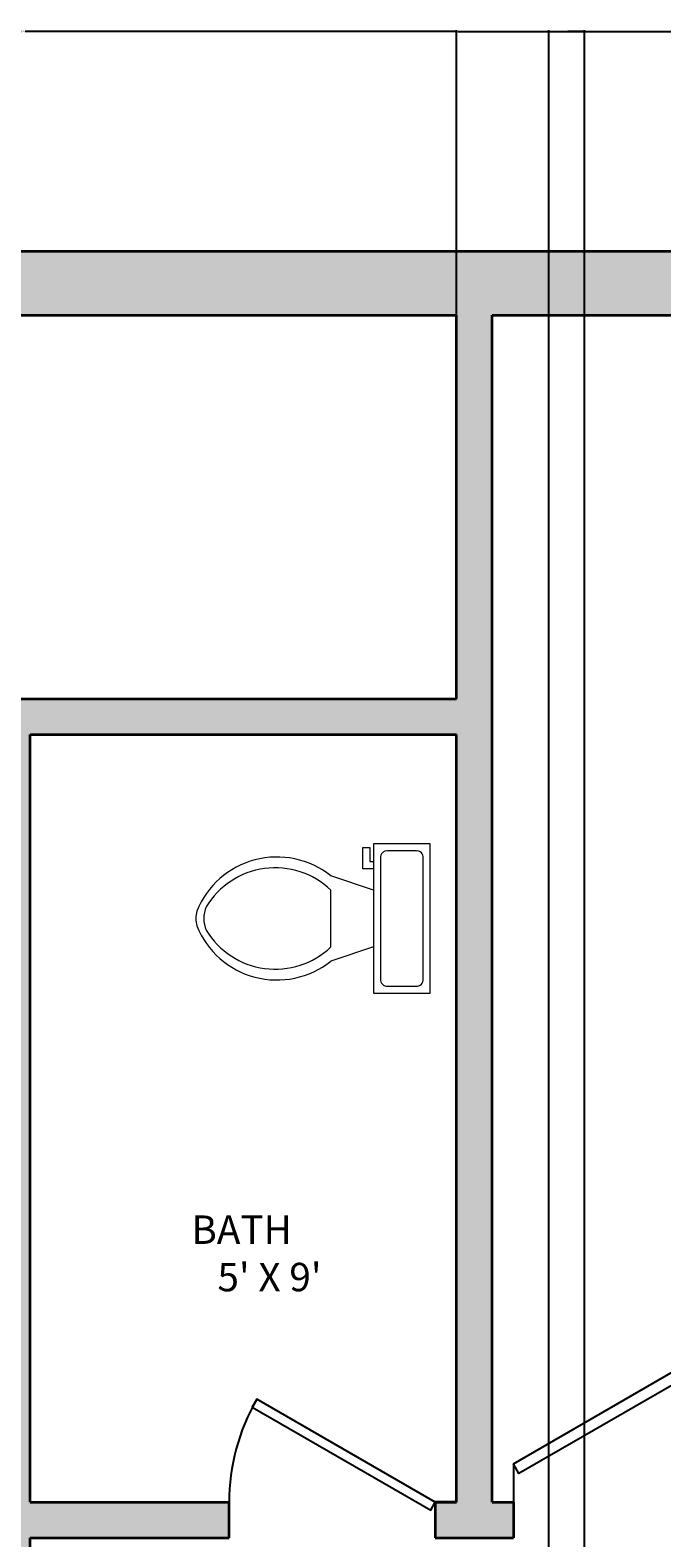
# Model space of a CAD drawing. Units: inches. Extents: x -30 to 437, y -29 to 647.
# Tile 14 of 15: x 187 to 276, y 435 to 647. Entities that reach past the tile are written whole.
import ezdxf

# ---------------------------------------------------------------- set-up
doc = ezdxf.new("R2010")
doc.units = ezdxf.units.IN
doc.header["$MEASUREMENT"] = 0
for name, color, linetype, lineweight in [('A-ANNO-DIMS', 2, 'Continuous', 18), ('A-AREA-IDEN', 7, 'Continuous', 18), ('A-WALL', 7, 'Continuous', 35), ('bathroom', 90, 'Continuous', 18), ('doors', 40, 'Continuous', 25)]:
    doc.layers.add(name, color=color, linetype=linetype, lineweight=lineweight)
doc.layers.add('A-WALL-PATT', color=251, linetype='Continuous', lineweight=13, true_color=0x636466)
doc.styles.get("Standard").update_dxf_attribs({"font": 'arial.ttf'})
doc.dimstyles.get("Standard").update_dxf_attribs({"dimtxt": 0.18, "dimasz": 0.18, "dimexe": 0.18, "dimexo": 0.0625, "dimgap": 0.09, "dimtad": 0, "dimtih": 1, "dimtoh": 1, "dimdec": 4, "dimzin": 0, "dimdsep": 46, "dimtxsty": 'Standard', "dimcen": 0.09, "dimadec": 0, "dimazin": 0, "dimtfac": 1, "dimtdec": 4, "dimtofl": 0, "dimtmove": 0, "dimatfit": 3, "dimfxl": 1, "dimtolj": 1, "dimtzin": 0, "dimarcsym": 0})

# ---------------------------------------------------------------- blocks, each defined once
blk = doc.blocks.new('Toilet - top')
for p, q in [((9.5, -6), (9.5, -2)), ((-8, -8.5), (-8, -8)), ((-7, -8), (-7, -9.5)), ((-4, -8), (-6, -14)), ((4, -8), (6, -14)), ((-10, -8.5), (-8, -8.5)), ((-10, -9.5), (-10, -8.5)), ((-7, -9.5), (-10, -9.5)), ((4, -14), (-4, -14))]:
    blk.add_line(p, q)
blk.add_lwpolyline([(10.5, -8), (10.5, 0), (-10.5, 0), (-10.5, -8)], close=True)
for points in [[(-9.5, -2), (-9.5, -6)], [(8.5, -1), (-8.5, -1)], [(-8.5, -7), (8.5, -7)]]:
    blk.add_lwpolyline(points)
for centre, radius, start, end in [((-8.62, -1.88), 0.884, 81.8699, 188.1301), ((8.62, -1.88), 0.884, 351.8699, 98.1301), ((-8.62, -6.12), 0.884, 171.8699, 278.1301), ((8.62, -6.12), 0.884, 261.8699, 8.1301), ((3.52, -21.58), 12.17, 141.4691, 247.9714), ((4.2, -21.82), 11.33, 136.3677, 238.9468), ((-3.52, -21.58), 12.17, 292.0284, 38.5307), ((-4.2, -21.82), 11.33, 301.053, 43.6321), ((0, -27.88), 4, 245.7318, 294.2682), ((0, -29), 4, 254.8605, 285.1395)]:
    blk.add_arc(centre, radius, start, end)
blk = doc.blocks.new('*U6')
for p, q in [((0, 0), (0, -6)), ((40, 0), (40, -6))]:
    blk.add_line(p, q)
blk.add_lwpolyline([(0, 0), (34.64, 20), (35.52, 18.48), (0.87, -1.52)], close=True)
blk.add_arc((0, 0), 40, 0, 30)
blk = doc.blocks.new('*U7')
for p, q in [((0, 0), (0, 6)), ((40, 0), (40, 6))]:
    blk.add_line(p, q)
blk.add_lwpolyline([(0, 0), (34.64, -20), (35.52, -18.48), (0.87, 1.52)], close=True)
blk.add_arc((0, 0), 40, 330, 0)
blk = doc.blocks.new('*D28')
at = {"layer": 'A-ANNO-DIMS', "color": 0, "lineweight": -2, "transparency": 16777216}
for p, q in [((124.67, 606.61), (124.67, 646.63)), ((124.85, 646.45), (185.39, 646.45)), ((246.49, 646.45), (185.95, 646.45)), ((246.67, 606.61), (246.67, 646.63))]:
    blk.add_line(p, q, dxfattribs=at)
at = {"layer": 'A-ANNO-DIMS', "color": 0, "transparency": 16777216}
for points in [[(124.85, 646.48), (124.85, 646.42), (124.67, 646.45)], [(246.49, 646.48), (246.49, 646.42), (246.67, 646.45)]]:
    blk.add_solid(points, dxfattribs=at)
at = {"layer": 'Defpoints', "color": 0, "transparency": 16777216}
for p in [(246.67, 646.45), (124.67, 606.55), (246.67, 606.55)]:
    blk.add_point(p, dxfattribs=at)
at = {"layer": 'A-ANNO-DIMS', "color": 0, "transparency": 16777216, "insert": (185.67, 646.45), "char_height": 0.18, "attachment_point": 5}
blk.add_mtext('\\A1;122', dxfattribs=at)
blk = doc.blocks.new('*D29')
at = {"layer": 'A-ANNO-DIMS', "color": 0, "lineweight": -2, "transparency": 16777216}
for p, q in [((246.67, 606.61), (246.67, 646.63)), ((246.85, 646.45), (325.89, 646.45)), ((405.49, 646.45), (326.45, 646.45)), ((405.67, 615.61), (405.67, 646.63))]:
    blk.add_line(p, q, dxfattribs=at)
at = {"layer": 'A-ANNO-DIMS', "color": 0, "transparency": 16777216}
for points in [[(246.85, 646.48), (246.85, 646.42), (246.67, 646.45)], [(405.49, 646.48), (405.49, 646.42), (405.67, 646.45)]]:
    blk.add_solid(points, dxfattribs=at)
at = {"layer": 'Defpoints', "color": 0, "transparency": 16777216}
for p in [(405.67, 646.45), (405.67, 615.55), (246.67, 606.55)]:
    blk.add_point(p, dxfattribs=at)
at = {"layer": 'A-ANNO-DIMS', "color": 0, "transparency": 16777216, "insert": (326.17, 646.45), "char_height": 0.18, "attachment_point": 5}
blk.add_mtext('\\A1;159', dxfattribs=at)
blk = doc.blocks.new('*D54')
at = {"layer": 'A-ANNO-DIMS', "color": 0, "lineweight": -2, "transparency": 16777216}
for p, q in [((259.67, 254.61), (259.67, 646.63)), ((259.85, 646.45), (262.02, 646.45)), ((264.49, 646.45), (262.32, 646.45)), ((264.67, 249.61), (264.67, 646.63))]:
    blk.add_line(p, q, dxfattribs=at)
at = {"layer": 'A-ANNO-DIMS', "color": 0, "transparency": 16777216}
for points in [[(259.85, 646.48), (259.85, 646.42), (259.67, 646.45)], [(264.49, 646.48), (264.49, 646.42), (264.67, 646.45)]]:
    blk.add_solid(points, dxfattribs=at)
at = {"layer": 'Defpoints', "color": 0, "transparency": 16777216}
for p in [(259.67, 646.45), (259.67, 254.55), (264.67, 249.55)]:
    blk.add_point(p, dxfattribs=at)
at = {"layer": 'A-ANNO-DIMS', "color": 0, "transparency": 16777216, "insert": (262.17, 646.45), "char_height": 0.18, "attachment_point": 5}
blk.add_mtext('\\A1;5', dxfattribs=at)

msp = doc.modelspace()

# ---------------------------------------------------------------- hatches: boundary and pattern name
at = {"layer": 'A-WALL-PATT'}
h = msp.add_hatch(color=256, dxfattribs=at)
h.dxf.hatch_style = 1
h.paths.add_polyline_path([(393.6054, 183.2352), (369.6054, 183.2352), (369.6054, 213.2352), (393.6054, 213.2352), (393.6054, 207.2352), (394.6054, 207.2352), (394.6054, 211.2352), (395.6054, 211.2352), (395.6054, 185.2352), (394.6054, 185.2352), (394.6054, 189.2352), (393.6054, 189.2352)], flags=0)
h.paths.add_polyline_path([(384.6054, 189.2352, -1), (390.6054, 189.2352, -1)], flags=0)
h.paths.add_polyline_path([(385.6054, 189.2352, -1), (389.6054, 189.2352, -1)], flags=0)
h.paths.add_polyline_path([(374.6054, 189.2352, -1), (382.6054, 189.2352, -1)], flags=0)
h.paths.add_polyline_path([(386.6054, 189.2352, -1), (388.6054, 189.2352, -1)], flags=0)
h.paths.add_polyline_path([(375.6054, 189.2352, -1), (381.6054, 189.2352, -1)], flags=0)
h.paths.add_polyline_path([(376.6054, 189.2352, -1), (380.6054, 189.2352, -1)], flags=0)
h.paths.add_polyline_path([(377.6054, 189.2352, -1), (379.6054, 189.2352, -1)], flags=0)
h.paths.add_polyline_path([(390.6054, 195.2352), (374.6054, 195.2352), (374.6054, 201.2352), (390.6054, 201.2352)], flags=0)
h.paths.add_polyline_path([(389.6054, 196.2352), (375.6054, 196.2352), (375.6054, 200.2352), (389.6054, 200.2352)], flags=0)
h.paths.add_polyline_path([(383.6054, 207.2352, -1), (391.6054, 207.2352, -1)], flags=0)
h.paths.add_polyline_path([(384.6054, 207.2352, -1), (390.6054, 207.2352, -1)], flags=0)
h.paths.add_polyline_path([(385.6054, 207.2352, -1), (389.6054, 207.2352, -1)], flags=0)
h.paths.add_polyline_path([(386.6054, 207.2352, -1), (388.6054, 207.2352, -1)], flags=0)
h.paths.add_polyline_path([(375.6054, 207.2352, -1), (381.6054, 207.2352, -1)], flags=0)
h.paths.add_polyline_path([(376.6054, 207.2352, -1), (380.6054, 207.2352, -1)], flags=0)
h.paths.add_polyline_path([(377.6054, 207.2352, -1), (379.6054, 207.2352, -1)], flags=0)
h.paths.add_polyline_path([(305.5437, 160.3663, -0.41421356), (304.0437, 158.8663), (271.0437, 158.8663, -0.41421356), (269.5437, 160.3663), (269.5437, 178.3663, -0.41421356), (271.0437, 179.8663), (304.0437, 179.8663, -0.41421356), (305.5437, 178.3663)], flags=0)
h.paths.add_polyline_path([(304.0437, 165.3663, -0.41421356), (303.0437, 164.3663), (289.2937, 164.3663, -0.41421356), (288.2937, 165.3663), (288.2937, 177.3663, -0.41421356), (289.2937, 178.3663), (303.0437, 178.3663, -0.41421356), (304.0437, 177.3663)], flags=0)
h.paths.add_polyline_path([(296.5437, 171.3663, -1), (295.5437, 171.3663, -1)], flags=0)
h.paths.add_polyline_path([(286.7937, 165.3663, -0.41421356), (285.7937, 164.3663), (272.0437, 164.3663, -0.41421356), (271.0437, 165.3663), (271.0437, 177.3663, -0.41421356), (272.0437, 178.3663), (285.7937, 178.3663, -0.41421356), (286.7937, 177.3663)], flags=0)
h.paths.add_polyline_path([(279.5437, 171.3663, -1), (278.5437, 171.3663, -1)], flags=0)
h.paths.add_polyline_path([(360.6737, 290.5474), (360.6737, 300.5474), (396.6737, 300.5474), (396.6737, 290.5474)], flags=0)
h.paths.add_polyline_path([(259.6737, 124.5474), (259.6737, 114.5474), (171.6737, 114.5474), (171.6737, 124.5474)], flags=0)
h.paths.add_polyline_path([(288.0737, 215.3705), (286.7097, 214.583), (268.7097, 245.7599), (270.0737, 246.5474)], flags=0)
h.paths.add_polyline_path([(259.6737, 168.5474), (256.6737, 168.5474), (256.6737, 173.5474), (256.6737, 179.0224), (255.8753, 177.6395), (224.2956, 195.872, 0.12053744), (220.1737, 179.0224, 0.12053744), (216.0518, 195.872), (184.4721, 177.6395), (183.6737, 179.0224), (215.2836, 197.2724), (216.0821, 195.8895), (216.0518, 195.872, -0.12053744), (220.1737, 179.0224, -0.12053744), (224.2956, 195.872), (224.2653, 195.8895), (225.0638, 197.2724), (256.6737, 179.0224), (256.6737, 173.5474), (259.6737, 173.5474)], flags=0)
h.paths.add_polyline_path([(386.7943, 325.4601), (372.6871, 325.4601), (372.6871, 339.5673), (386.7943, 339.5673)], flags=0)
h.paths.add_polyline_path([(359.5875, 343.7429), (357.7905, 343.7429), (357.7905, 327.9179), (359.3933, 327.9179, 0.41420885), (361.5302, 330.0549), (361.5302, 341.8434, 0.41436161)], flags=0)
h.paths.add_polyline_path([(341.7887, 323.1235, -0.11921667), (340.7839, 323.1235)], flags=0)
h.paths.add_polyline_path([(379.6332, 328.8632), (379.6332, 332.2699), (376.0992, 332.2699, 0.39427733)], flags=0)
h.paths.add_polyline_path([(375.5299, 332.459, -1), (383.8511, 332.459, -1)], flags=0)
h.paths.add_polyline_path([(388.9363, 344.7425), (372.5309, 344.7425, -0.41421356), (370.394, 346.8794), (370.394, 347.5594, -0.39085173), (372.3472, 349.7005, -0.43951011), (370.394, 351.4933), (370.394, 365.1894, -0.40305452), (372.2191, 367.1298, -0.41839453), (370.394, 368.9291), (370.394, 382.6251, -0.40885826), (372.2519, 384.5722, -0.42377324), (370.394, 386.3707), (370.394, 400.0667, -0.38660687), (372.1327, 402.0094), (372.531, 402.0094, -0.41421834), (370.394, 404.1464), (370.394, 404.7778, -0.41420891), (372.5309, 406.9147), (388.9363, 406.9147, -0.41421821), (391.0733, 404.7778), (391.0733, 346.8794, -0.41421356)], flags=0)
edge = h.paths.add_edge_path(flags=0)
edge.add_spline(control_points=[(349.3585, 363.204), (349.0859, 363.204), (348.8133, 363.2227), (348.2712, 363.2973), (348.0016, 363.3531), (347.3533, 363.5328), (346.9776, 363.6755), (346.2445, 364.0308), (345.887, 364.2432), (345.1953, 364.7329), (344.8611, 365.0101), (344.2197, 365.6237), (343.9125, 365.9603), (343.211, 366.8336), (342.8313, 367.3965), (342.1401, 368.6117), (341.8286, 369.2641), (341.2807, 370.64), (341.0443, 371.3636), (340.6522, 372.8619), (340.4964, 373.6367), (340.2695, 375.2158), (340.1983, 376.0203), (340.142, 377.6365), (340.157, 378.4483), (340.2729, 380.0567), (340.3738, 380.8533), (340.6589, 382.4093), (340.8432, 383.1686), (341.2906, 384.629), (341.5538, 385.3301), (342.1531, 386.6544), (342.4891, 387.2776), (343.2266, 388.4288), (343.6281, 388.9567), (344.4879, 389.9012), (344.9463, 390.3178), (345.7981, 390.9428), (346.182, 391.1771), (346.9712, 391.5648), (347.3766, 391.7182), (348.2004, 391.9387), (348.6189, 392.0058), (349.4588, 392.0508), (349.8801, 392.0288), (350.7146, 391.8966), (351.1278, 391.7865), (351.9366, 391.4822), (352.3323, 391.2882), (353.0989, 390.8223), (353.4699, 390.5504), (354.1819, 389.9355), (354.5229, 389.5924), (355.1706, 388.8418), (355.4772, 388.4343), (356.1315, 387.4422), (356.4671, 386.8397), (357.0692, 385.5581), (357.3356, 384.879), (357.7933, 383.4624), (357.9846, 382.725), (358.2875, 381.2112), (358.3992, 380.4349), (358.5404, 378.8643), (358.5699, 378.0699), (358.546, 376.4841), (358.4926, 375.6928), (358.3042, 374.1343), (358.1692, 373.3672), (357.8207, 371.8774), (357.6072, 371.1549), (357.1067, 369.7735), (356.8196, 369.1148), (356.1782, 367.8787), (355.8238, 367.3013), (355.0551, 366.244), (354.6408, 365.7641), (353.7607, 364.9161), (353.2948, 364.5481), (352.445, 364.0149), (352.0701, 363.822), (351.3034, 363.5117), (350.9116, 363.3943), (350.1325, 363.2418), (349.7455, 363.204), (349.3585, 363.204)], knot_values=[3.14159265, 3.14159265, 3.14159265, 3.14159265, 3.22691715, 3.22691715, 3.31224165, 3.31224165, 3.43426671, 3.43426671, 3.55629177, 3.55629177, 3.67831683, 3.67831683, 3.8003419, 3.8003419, 3.97157384, 3.97157384, 4.14280577, 4.14280577, 4.31403771, 4.31403771, 4.48526965, 4.48526965, 4.65650159, 4.65650159, 4.82773353, 4.82773353, 4.99896547, 4.99896547, 5.1701974, 5.1701974, 5.34142934, 5.34142934, 5.51266128, 5.51266128, 5.68389322, 5.68389322, 5.85512516, 5.85512516, 5.98669107, 5.98669107, 6.11825699, 6.11825699, 6.24982291, 6.24982291, 6.38138882, 6.38138882, 6.51295474, 6.51295474, 6.64452065, 6.64452065, 6.77608657, 6.77608657, 6.90765249, 6.90765249, 7.0392184, 7.0392184, 7.20701563, 7.20701563, 7.37481286, 7.37481286, 7.54261009, 7.54261009, 7.71040732, 7.71040732, 7.87820455, 7.87820455, 8.04600178, 8.04600178, 8.21379901, 8.21379901, 8.38159624, 8.38159624, 8.54939347, 8.54939347, 8.7171907, 8.7171907, 8.88498794, 8.88498794, 9.05278517, 9.05278517, 9.17820699, 9.17820699, 9.30362881, 9.30362881, 9.42477796, 9.42477796, 9.42477796, 9.42477796], degree=3, periodic=0)
edge.add_line((341.1696, 384.3006), (341.2012, 384.2808))
edge = h.paths.add_edge_path(flags=0)
edge.add_line((344.3353, 388.7801), (344.317, 388.7915))
edge.add_ellipse((349.3585, 377.6204), major_axis=(0, -13.7895), ratio=0.62186025, start_angle=-244.867444, end_angle=-124.769923)
h.paths.add_polyline_path([(163.6737, 163.1474), (132.4968, 145.1474), (131.7093, 146.5114), (162.8862, 164.5114)], flags=0)
h.paths.add_polyline_path([(366.4355, 409.0896, -0.41423669), (364.2985, 406.9525, -0.4913499), (361.5302, 408.8973), (361.5302, 420.6405, 0.41421356), (359.3932, 422.7775), (357.7905, 422.7775), (357.7905, 406.9525), (359.6317, 406.9525, 0.42741026), (361.5332, 408.9757, 0.39869469), (363.6672, 406.9525, 0.51958103), (366.4355, 409.0895)], flags=0)
h.paths.add_polyline_path([(386.7943, 410.9671), (372.6871, 410.9671), (372.6871, 425.0742), (386.7943, 425.0742)], flags=0)
h.paths.add_polyline_path([(379.6332, 414.3701), (379.6332, 417.7768), (376.0992, 417.7768, 0.39427733)], flags=0)
h.paths.add_polyline_path([(375.5299, 417.966, -1), (383.8511, 417.966, -1)], flags=0)
h.paths.add_polyline_path([(150.0377, 351.583), (148.6737, 352.3705), (166.6737, 383.5474), (168.0377, 382.7599)], flags=0)
h.paths.add_polyline_path([(91.6737, 234.1974), (66.559, 219.6974), (65.9246, 220.7962), (91.0393, 235.2962)], flags=0)
h.paths.add_polyline_path([(255.4612, 443.5834), (254.6737, 444.9474), (285.8506, 462.9474), (286.6381, 461.5834)], flags=0)
h.paths.add_polyline_path([(176.2737, 394.5474), (158.2737, 425.7243), (159.6377, 426.5118), (177.6377, 395.3349)], flags=0)
h.paths.add_polyline_path([(243.6737, 439.5474), (243.0393, 438.4486), (217.9246, 452.9486), (218.559, 454.0474)], flags=0)
h.paths.add_polyline_path([(38.1264, 269.8429), (40.2408, 269.8429), (40.2408, 270.3508), (38.1264, 270.3508)], flags=0)
h.paths.add_polyline_path([(75.7157, 289.9439), (40.2408, 289.9439), (38.1264, 289.6524), (40.2408, 289.6524)], flags=0)
h.paths.add_polyline_path([(75.7157, 270.0846), (77.6447, 270.0846), (77.6697, 270.1626), (75.7175, 270.1626)], flags=0)
h.paths.add_polyline_path([(80.5373, 293.3002), (33.0467, 293.3002), (13.5054, 293.3002), (13.5054, 351.9244), (29.7898, 351.9244), (80.5373, 351.9244)], flags=0)
h.paths.add_polyline_path([(46.0261, 212.466, -0.50131678), (27.1651, 207.5106), (21.165, 209.5107), (21.165, 206.5107), (22.665, 206.5107), (22.665, 203.5107), (21.165, 203.5107), (21.165, 203.0107), (13.165, 203.0107), (13.165, 224.0107), (21.165, 224.0107), (21.165, 217.5107), (27.1649, 219.5106, -0.50132349), (46.0261, 214.5554, -0.13289091)], flags=0)
h.paths.add_polyline_path([(44.688, 211.8666, -0.48007965), (27.165, 209.5107), (27.165, 217.5107, -0.4800795), (44.688, 215.1547, -0.21500378)], flags=0)
h.paths.add_polyline_path([(19.415, 204.0107), (15.165, 204.0107, -0.41421356), (14.165, 204.7607), (14.165, 222.0107, -0.41421356), (14.915, 223.0107), (19.165, 223.0107, -0.41421356), (20.165, 222.2607), (20.165, 205.0107, -0.41421356)], flags=0)
h.paths.add_polyline_path([(32.7608, 269.0719), (31.8439, 269.0719), (31.8439, 268.6134), (13.5054, 268.6134), (13.5054, 291.5366), (31.8439, 291.5366), (32.7608, 291.0781), (32.7608, 280.9919, -1), (32.7608, 279.1581)], flags=0)
h.paths.add_polyline_path([(40.2408, 360.1436), (38.1264, 360.1436), (38.1264, 359.6357), (40.2408, 359.6357)], flags=0)
h.paths.add_polyline_path([(75.7157, 355.2807), (40.2408, 355.2807), (38.1264, 355.5722), (40.2408, 355.5722), (40.2408, 355.2807), (75.7157, 355.2807), (75.7157, 375.5982), (40.2408, 375.5982), (38.1264, 375.3817), (40.2408, 375.3817), (40.2408, 375.5982), (75.7157, 375.5982), (77.9733, 375.062), (75.7175, 375.062), (75.7175, 374.554)], flags=0)
h.paths.add_polyline_path([(42.8174, 299.814, 0.13867074), (34.1602, 294.603), (14.8081, 294.603), (14.8081, 350.6216), (29.8539, 350.6216, 0.09822056)], flags=0)
h.paths.add_polyline_path([(15.8636, 276.7781, -0.30640166), (20.3757, 283.4499), (20.3483, 290.6726), (31.4014, 290.7146), (31.4309, 282.9124), (26.8287, 282.895, -0.26006276), (30.241, 276.7781, -1)], flags=0)
h.paths.add_polyline_path([(26.1332, 276.7781), (23.0523, 273.6972), (19.9714, 276.7781), (23.0523, 279.8589), (23.0523, 283.9209), (21.3493, 283.9145), (20.7006, 283.5219), (20.6907, 286.1226), (23.2914, 286.1325), (25.8936, 285.7522), (27.1939, 285.7572), (28.4928, 286.1522), (31.0935, 286.1621), (31.0918, 286.6172), (25.6303, 286.5965), (25.616, 290.3675), (31.0775, 290.3882), (31.0918, 286.6172), (31.1034, 283.5614), (28.5027, 283.5515), (25.9005, 283.9317), (23.0523, 283.9209), (23.0523, 279.8589)], flags=0)
h.paths.add_polyline_path([(24.0793, 276.7781, -1), (22.0253, 276.7781, -1)], flags=0)
h.paths.add_polyline_path([(35.7687, 302.2895, -0.41421356), (35.2283, 301.2726), (22.2164, 297.2909, -0.41421356), (21.1995, 297.8313), (15.7317, 315.6996, -0.41421356), (16.2721, 316.7165), (18.8554, 317.507), (15.3721, 328.8904, -0.41421356), (15.9125, 329.9073), (28.9244, 333.889, -0.41421356), (29.9414, 333.3486), (35.4091, 315.4802, -0.41421356), (34.8687, 314.4633), (32.2854, 313.6728)], flags=0)
h.paths.add_polyline_path([(361.3728, 532.6207), (302.7487, 532.6207), (302.7487, 580.1113), (302.7487, 599.6527), (361.3728, 599.6527), (361.3728, 583.3682)], flags=0)
h.paths.add_polyline_path([(370.1, 575.0316), (370.1, 572.9172), (370.6079, 572.9172), (370.6079, 575.0316)], flags=0)
h.paths.add_polyline_path([(385.0466, 537.4423), (385.0466, 572.9172), (384.8302, 575.0316), (384.8302, 572.9172)], flags=0)
h.paths.add_polyline_path([(384.5104, 535.3262), (384.5104, 537.4406), (384.0025, 537.4406), (364.7291, 537.4423), (364.7291, 572.9172), (365.0206, 575.0316), (365.0206, 572.9172), (364.7291, 572.9172), (364.7291, 537.4423), (384.5884, 537.4423), (384.5884, 535.5133)], flags=0)
h.paths.add_polyline_path([(384.5884, 535.5133), (383.4945, 535.164), (383.4945, 537.4406), (382.9866, 535.3262), (382.9866, 537.4406), (383.4945, 535.3262), (383.4945, 537.4406), (384.5884, 537.4406)], flags=0)
h.paths.add_polyline_path([(23.874, 286.8174), (21.0132, 286.8065), (21.0004, 290.1875), (23.8612, 290.1983)], flags=0)
h.paths.add_polyline_path([(242.9824, 511.1667), (234.9824, 511.1667), (234.9824, 517.6667), (228.9825, 515.6667, -0.50132349), (210.1213, 520.622, -0.13289091), (210.1213, 522.7114, -0.50131678), (228.9823, 527.6667), (234.9824, 525.6667), (234.9824, 528.6667), (233.4824, 528.6667), (233.4824, 531.6667), (234.9824, 531.6667), (234.9824, 532.1667), (242.9824, 532.1667)], flags=0)
h.paths.add_polyline_path([(236.9824, 512.1667, -0.41421356), (235.9824, 512.9167), (235.9824, 530.1667, -0.41421356), (236.7324, 531.1667), (240.9824, 531.1667, -0.41421356), (241.9824, 530.4167), (241.9824, 513.1667, -0.41421356), (241.2324, 512.1667)], flags=0)
h.paths.add_polyline_path([(279.533, 537.4423), (279.533, 535.5133), (279.6111, 535.4884), (279.6111, 537.4406)], flags=0)
h.paths.add_polyline_path([(279.2913, 575.0316), (279.2913, 572.9172), (279.7992, 572.9172), (279.7992, 575.0316)], flags=0)
h.paths.add_polyline_path([(211.4594, 520.0227, -0.21500378), (211.4594, 523.3107, -0.48007965), (228.9824, 525.6667), (228.9824, 517.6667, -0.4800795)], flags=0)
h.paths.add_polyline_path([(32.7627, 354.1465), (31.8457, 354.1465), (31.8457, 353.688), (13.5054, 353.688), (13.5054, 376.6134), (31.8457, 376.6134), (32.7627, 376.1549), (32.7627, 366.0677, -1), (32.7627, 364.2337)], flags=0)
h.paths.add_polyline_path([(15.9446, 365.1507, -1), (30.3234, 365.1507, -1)], flags=0)
h.paths.add_polyline_path([(41.213, 428.467), (43.3274, 428.467), (43.3274, 428.9749), (41.213, 428.9749)], flags=0)
h.paths.add_polyline_path([(78.8022, 448.568), (43.3274, 448.568), (41.213, 448.2765), (43.3274, 448.2765)], flags=0)
h.paths.add_polyline_path([(78.8022, 428.7087), (80.7313, 428.7087), (80.7562, 428.7868), (78.804, 428.7868)], flags=0)
h.paths.add_polyline_path([(26.2152, 365.1507), (23.134, 362.0696), (20.0529, 365.1507), (23.134, 368.2319)], flags=0)
h.paths.add_polyline_path([(24.1611, 365.1507, -1), (22.107, 365.1507, -1)], flags=0)
h.paths.add_polyline_path([(309.2625, 570.3406, 0.13867074), (304.0514, 578.9978), (304.0514, 598.3499), (360.07, 598.3499), (360.07, 583.3041, 0.09822056)], flags=0)
h.paths.add_polyline_path([(246.6737, 552.5474), (129.6737, 552.5474), (129.6737, 606.5474), (246.6737, 606.5474)], flags=16)
h.paths.add_polyline_path([(373.6822, 580.3953), (363.595, 580.3953), (363.595, 581.3123), (363.1365, 581.3123), (363.1365, 599.6527), (386.0619, 599.6527), (386.0619, 581.3123), (385.6034, 580.3953), (375.5162, 580.3953, -1)], flags=0)
h.paths.add_polyline_path([(83.6239, 451.9244), (36.1333, 451.9244), (16.5919, 451.9244), (16.5919, 510.5485), (32.8764, 510.5485), (83.6239, 510.5485)], flags=0)
h.paths.add_polyline_path([(367.4098, 590.024, -1), (381.7886, 590.024, -1)], flags=0)
h.paths.add_polyline_path([(374.5992, 586.9428), (371.518, 590.024), (374.5992, 593.1052), (377.6803, 590.024)], flags=0)
h.paths.add_polyline_path([(373.5721, 590.024, -1), (375.6262, 590.024, -1)], flags=0)
h.paths.add_polyline_path([(324.9287, 577.7489, -0.41421356), (323.9118, 578.2893), (323.1212, 580.8726), (311.7379, 577.3893, -0.41421356), (310.721, 577.9297), (306.7393, 590.9416, -0.41421356), (307.2797, 591.9585), (325.1481, 597.4263, -0.41421356), (326.165, 596.8859), (326.9555, 594.3026), (338.3388, 597.7859, -0.41421356), (339.3557, 597.2455), (343.3374, 584.2336, -0.41421356), (342.797, 583.2167)], flags=0)
h.paths.add_polyline_path([(300.5265, 580.3972), (290.4404, 580.3972, -1), (288.6065, 580.3972), (278.5203, 580.3972), (278.5203, 581.3142), (278.0619, 581.3142), (278.0619, 599.6527), (300.985, 599.6527), (300.985, 581.3142)], flags=0)
h.paths.add_polyline_path([(300.163, 581.7567), (292.3609, 581.7271), (292.3434, 586.3294, -0.75567924), (279.0378, 590.1057, -0.82536731), (292.8983, 592.7823), (300.1211, 592.8097)], flags=0)
h.paths.add_polyline_path([(299.8367, 582.0805), (296.0656, 582.0662), (293.0098, 582.0546), (292.9999, 584.6553), (293.3802, 587.2575), (293.3694, 590.1057), (289.3074, 590.1057), (286.2265, 587.0248), (283.1456, 590.1057), (286.2265, 593.1866), (289.3074, 590.1057), (293.3694, 590.1057), (293.3629, 591.8088), (292.9703, 592.4575), (295.5711, 592.4673), (295.5809, 589.8666), (295.2007, 587.2644), (295.2056, 585.9641), (295.6006, 584.6652), (295.6105, 582.0645), (296.0656, 582.0662), (296.0449, 587.5277), (299.8159, 587.542)], flags=0)
h.paths.add_polyline_path([(285.1995, 590.1057, -1), (287.2535, 590.1057, -1)], flags=0)
h.paths.add_polyline_path([(299.6467, 589.2969), (296.2658, 589.284), (296.255, 592.1448), (299.6359, 592.1576)], flags=0)
h.paths.add_polyline_path([(35.8473, 427.696), (34.9304, 427.696), (34.9304, 427.2376), (16.5919, 427.2376), (16.5919, 450.1607), (34.9304, 450.1607), (35.8473, 449.7022), (35.8473, 439.6161, -1), (35.8473, 437.7822)], flags=0)
h.paths.add_polyline_path([(18.9502, 435.4022, -0.30640166), (23.4623, 442.074), (23.4349, 449.2968), (34.4879, 449.3387), (34.5175, 441.5366), (29.9152, 441.5191, -0.26006276), (33.3275, 435.4022, -1)], flags=0)
h.paths.add_polyline_path([(29.2197, 435.4022), (26.1389, 432.3213), (23.058, 435.4022), (26.1389, 438.4831), (26.1389, 442.5451), (24.4358, 442.5386), (23.7871, 442.1461), (23.7772, 444.7468), (26.378, 444.7566), (28.9801, 444.3764), (30.2805, 444.3813), (31.5794, 444.7764), (34.1801, 444.7862), (34.1784, 445.2413), (28.7169, 445.2206), (28.7026, 448.9917), (34.164, 449.0124), (34.1784, 445.2413), (34.1899, 442.1855), (31.5892, 442.1756), (28.987, 442.5559), (26.1389, 442.5451), (26.1389, 438.4831)], flags=0)
h.paths.add_polyline_path([(27.1658, 435.4022, -1), (25.1119, 435.4022, -1)], flags=0)
h.paths.add_polyline_path([(45.904, 458.4382, 0.13867074), (37.2467, 453.2271), (17.8947, 453.2271), (17.8947, 509.2457), (32.9405, 509.2457, 0.09822056)], flags=0)
h.paths.add_polyline_path([(26.9605, 445.4415), (24.0997, 445.4307), (24.0869, 448.8116), (26.9477, 448.8225)], flags=0)
h.paths.add_polyline_path([(38.3149, 459.8967), (25.3029, 455.915, -0.41421356), (24.286, 456.4554), (18.8183, 474.3238, -0.41421356), (19.3586, 475.3407), (21.942, 476.1312), (18.4587, 487.5145, -0.41421356), (18.999, 488.5314), (32.011, 492.5131, -0.41421356), (33.0279, 491.9727), (38.4957, 474.1044, -0.41421356), (37.9553, 473.0875), (35.3719, 472.297), (38.8553, 460.9136, -0.41421356)], flags=0)
h.paths.add_polyline_path([(43.3274, 518.7678), (41.213, 518.7678), (41.213, 518.2598), (43.3274, 518.2598)], flags=0)
h.paths.add_polyline_path([(78.8022, 513.9049), (43.3274, 513.9049), (41.213, 514.1964), (43.3274, 514.1964), (43.3274, 513.9049), (78.8022, 513.9049), (78.8022, 534.2223), (43.3274, 534.2223), (41.213, 534.0059), (43.3274, 534.0059), (43.3274, 534.2223), (78.8022, 534.2223), (81.0599, 533.6861), (78.804, 533.6861), (78.804, 533.1782)], flags=0)
h.paths.add_polyline_path([(121.6737, 556.8974), (121.0393, 555.7986), (95.9246, 570.2986), (96.559, 571.3974)], flags=0)
h.paths.add_polyline_path([(35.8493, 512.7707), (34.9322, 512.7707), (34.9322, 512.3122), (16.5919, 512.3122), (16.5919, 535.2376), (34.9322, 535.2376), (35.8493, 534.7791), (35.8493, 524.6919, -1), (35.8493, 522.8579)], flags=0)
h.paths.add_polyline_path([(19.0312, 523.7749, -1), (33.41, 523.7749, -1)], flags=0)
h.paths.add_polyline_path([(26.2206, 520.6937), (23.1394, 523.7749), (26.2206, 526.8561), (29.3018, 523.7749)], flags=0)
h.paths.add_polyline_path([(25.1935, 523.7749, -1), (27.2476, 523.7749, -1)], flags=0)
h.paths.add_polyline_path([(28.4381, 586.0173), (22.438, 588.0173), (22.438, 585.0173), (23.938, 585.0173), (23.938, 582.0173), (22.438, 582.0173), (22.438, 581.5173), (14.438, 581.5173), (14.438, 602.5173), (22.438, 602.5173), (22.438, 596.0173), (28.4379, 598.0173, -0.50132349), (47.2992, 593.062, -0.13289091), (47.2992, 590.9726, -0.50131678)], flags=0)
h.paths.add_polyline_path([(28.438, 588.0174), (28.438, 596.0173, -0.4800795), (45.961, 593.6614, -0.21500378), (45.961, 590.3733, -0.48007965)], flags=0)
h.paths.add_polyline_path([(20.688, 582.5173), (16.438, 582.5173, -0.41421356), (15.438, 583.2673), (15.438, 600.5173, -0.41421356), (16.188, 601.5173), (20.438, 601.5173, -0.41421356), (21.438, 600.7673), (21.438, 583.5173, -0.41421356)], flags=0)
h.paths.add_polyline_path([(171.6737, 2.0474), (171.6737, 104.5474), (259.6737, 104.5474), (259.6737, 148.5474), (396.6737, 148.5474), (396.6737, 2.0474), (405.6737, 2.0474), (405.6737, 615.5474), (1.6737, 615.5474), (1.6737, 2.0474)])
h.paths.add_polyline_path([(171.6737, 104.5474), (259.6737, 104.5474), (259.6737, 210.5474), (264.6737, 210.5474), (264.6737, 153.5474), (396.6737, 153.5474), (396.6737, 249.5474), (264.6737, 249.5474), (264.6737, 246.5474), (259.6737, 246.5474), (259.6737, 254.5474), (396.6737, 254.5474), (396.6737, 434.5474), (290.6737, 434.5474), (290.6737, 439.5474), (396.6737, 439.5474), (396.6737, 606.5474), (251.6737, 606.5474), (251.6737, 439.5474), (254.6737, 439.5474), (254.6737, 434.5474), (243.6737, 434.5474), (243.6737, 439.5474), (246.6737, 439.5474), (246.6737, 547.5474), (186.6737, 547.5474), (186.6737, 439.5474), (214.6737, 439.5474), (214.6737, 434.5474), (186.6737, 434.5474), (186.6737, 430.5474), (181.6737, 430.5474), (181.6737, 547.5474), (121.6737, 547.5474), (121.6737, 552.5474), (124.6737, 552.5474), (124.6737, 606.5474), (10.6737, 606.5474), (10.6737, 552.5474), (92.6737, 552.5474), (92.6737, 547.5474), (10.6737, 547.5474), (10.6737, 391.5474), (181.6737, 391.5474), (181.6737, 394.5474), (186.6737, 394.5474), (186.6737, 386.5474), (171.6737, 386.5474), (171.6737, 383.5474), (166.6737, 383.5474), (166.6737, 386.5474), (10.6737, 386.5474), (10.6737, 238.5474), (62.6737, 238.5474), (62.6737, 233.5474), (10.6737, 233.5474), (10.6737, 173.5474), (94.6737, 173.5474), (94.6737, 233.5474), (91.6737, 233.5474), (91.6737, 238.5474), (166.6737, 238.5474), (166.6737, 347.5474), (171.6737, 347.5474), (171.6737, 233.5474), (99.6737, 233.5474), (99.6737, 173.5474), (127.6737, 173.5474), (127.6737, 168.5474), (10.6737, 168.5474), (10.6737, 11.0474), (166.6737, 11.0474), (166.6737, 168.5474), (163.6737, 168.5474), (163.6737, 173.5474), (183.6737, 173.5474), (183.6737, 168.5474), (171.6737, 168.5474)])

# ---------------------------------------------------------------- linework, layer by layer
at = {"layer": 'A-WALL'}
for p, q in [((129.6737, 606.5474), (246.6737, 606.5474)), ((246.6737, 552.5474), (246.6737, 606.5474)), ((251.6737, 606.5474), (396.6737, 606.5474)), ((251.6737, 439.5474), (251.6737, 606.5474)), ((129.6737, 552.5474), (246.6737, 552.5474)), ((186.6737, 547.5474), (246.6737, 547.5474)), ((186.6737, 439.5474), (186.6737, 547.5474)), ((246.6737, 439.5474), (246.6737, 547.5474)), ((186.6737, 439.5474), (214.6737, 439.5474)), ((214.6737, 434.5474), (214.6737, 439.5474)), ((243.6737, 439.5474), (246.6737, 439.5474)), ((246.6737, 439.5474), (243.6737, 439.5474)), ((243.6737, 439.5474), (243.6737, 434.5474)), ((251.6737, 439.5474), (254.6737, 439.5474)), ((251.6737, 439.5474), (254.6737, 439.5474)), ((254.6737, 439.5474), (254.6737, 434.5474)), ((186.6737, 434.5474), (214.6737, 434.5474)), ((186.6737, 430.5474), (186.6737, 434.5474)), ((243.6737, 434.5474), (254.6737, 434.5474))]:
    msp.add_line(p, q, dxfattribs=at)
msp.add_lwpolyline([(171.6737, 2.0474), (1.6737, 2.0474), (1.6737, 615.5474), (405.6737, 615.5474), (405.6737, 2.0474), (396.6737, 2.0474)], dxfattribs=at)

# ---------------------------------------------------------------- block references
at = {"layer": 'bathroom', "rotation": 270}
msp.add_blockref('Toilet - top', (242.9824, 521.6667), dxfattribs=at)
at = {"layer": 'doors', "xscale": 0.8999999999999548, "yscale": 0.8999999999999548, "zscale": 0.8999999999999548}
msp.add_blockref('*U6', (254.6737, 444.9474), dxfattribs=at)
at = {"layer": 'doors', "xscale": 0.725, "yscale": 0.725, "zscale": 0.725, "rotation": 180}
msp.add_blockref('*U7', (243.6737, 439.5474), dxfattribs=at)

# ---------------------------------------------------------------- texts
at = {"layer": 'A-AREA-IDEN', "insert": (208.1364, 479.8973), "char_height": 4, "attachment_point": 1}
msp.add_mtext_dynamic_manual_height_columns(" BATH\\P    5' X 9'", width=25.99481, gutter_width=1, heights=[0], dxfattribs=at)

# ---------------------------------------------------------------- dimensions: what is measured, and where the dimension line sits
at = {"layer": 'A-ANNO-DIMS'}
for base, p1, p2, picture, middle in [((246.6737, 646.4474), (124.6737, 606.5474), (246.6737, 606.5474), '*D28', (185.6737, 646.4474)), ((405.6737, 646.4474), (246.6737, 606.5474), (405.6737, 615.5474), '*D29', (326.1737, 646.4474)), ((259.6737, 646.4474), (264.6737, 249.5474), (259.6737, 254.5474), '*D54', (262.1737, 646.4474))]:
    dim = msp.add_linear_dim(base=base, p1=p1, p2=p2, dimstyle='Standard', override={"dimdec": 0, "dimlfac": 1, "dimrnd": 0, "dimzin": 0, "dimdsep": 46, "dimlunit": 2}, dxfattribs=at)
    dim.commit()
    dim.dimension.update_dxf_attribs({"geometry": picture, "text_midpoint": middle})

doc.saveas('drawing.dxf')
